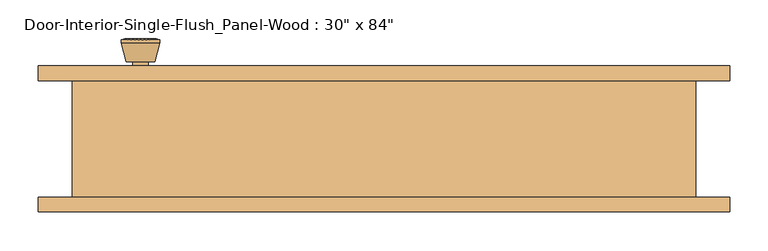
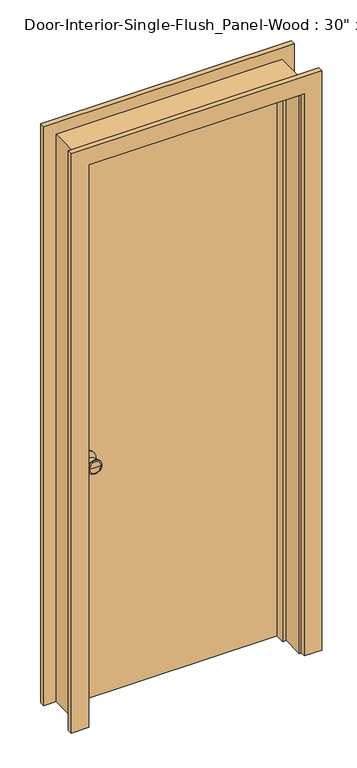
"""IFC4 building model written with IfcOpenShell, lengths in millimetres: door geometry."""

from ifc_helpers import new_model, si_unit, point, frame, frame_2d, origin, origin_with_axes, place, context, project, spatial, polyline, circle_curve, trimmed, segment, composite_curve, outline, extrude, faceted_brep, source, transform, mapped, element, save
from ifc_brep_helpers import plane_surface, cylinder_surface, revolved_surface, advanced_brep


def door_160b0797(model_context):
    return source(origin(), model_context, "Body", "SolidModel", [
        advanced_brep(
        [(-317.5, 32.1, 914.4), (-307.5, 32.1, 914.4), (-327.5, 32.1, 914.4), (-297.0241324, -16.9, 914.4), (-317.5, -16.9, 914.4), (-337.9758676, -16.9, 914.4), (-292.5, -15.0721319, 914.4), (-342.5, -15.0721319, 914.4), (-292.5, -11.6084537, 914.4), (-342.5, -11.6084537, 914.4), (-298.863764, 13.1, 914.4), (-336.136236, 13.1, 914.4), (-307.5, 13.1, 914.4), (-327.5, 13.1, 914.4)],
        [
            (0, 1),
            (1, 2, circle_curve(frame((-317.5, 32.1, 914.4), z_axis=(0.0, 1.0, 0.0), x_axis=(-1.0, 0.0, 0.0)), 10.0)),
            (2, 0),
            (2, 1, circle_curve(frame((-317.5, 32.1, 914.4), z_axis=(0.0, 1.0, 0.0), x_axis=(-1.0, 0.0, 0.0)), 10.0)),
            (3, 4),
            (4, 5),
            (5, 3, circle_curve(frame((-317.5, -16.9, 914.4), z_axis=(0.0, -1.0, 0.0), x_axis=(-1.0, 0.0, 0.0)), 20.4758676)),
            (3, 5, circle_curve(frame((-317.5, -16.9, 914.4), z_axis=(0.0, -1.0, 0.0), x_axis=(-1.0, 0.0, 0.0)), 20.4758676)),
            (6, 3),
            (5, 7),
            (7, 6, circle_curve(frame((-317.5, -15.0721319, 914.4), z_axis=(0.0, -1.0, 0.0), x_axis=(-1.0, 0.0, 0.0)), 25.0)),
            (6, 7, circle_curve(frame((-317.5, -15.0721319, 914.4), z_axis=(0.0, -1.0, 0.0), x_axis=(-1.0, 0.0, 0.0)), 25.0)),
            (8, 6),
            (7, 9),
            (9, 8, circle_curve(frame((-317.5, -11.6084537, 914.4), z_axis=(0.0, -1.0, 0.0), x_axis=(-1.0, 0.0, 0.0)), 25.0)),
            (8, 9, circle_curve(frame((-317.5, -11.6084537, 914.4), z_axis=(0.0, -1.0, 0.0), x_axis=(-1.0, 0.0, 0.0)), 25.0)),
            (10, 8),
            (9, 11),
            (11, 10, circle_curve(frame((-317.5, 13.1, 914.4), z_axis=(0.0, -1.0, 0.0), x_axis=(-1.0, 0.0, 0.0)), 18.636236)),
            (10, 11, circle_curve(frame((-317.5, 13.1, 914.4), z_axis=(0.0, -1.0, 0.0), x_axis=(-1.0, 0.0, 0.0)), 18.636236)),
            (12, 10),
            (11, 13),
            (13, 12, circle_curve(frame((-317.5, 13.1, 914.4), z_axis=(0.0, -1.0, 0.0), x_axis=(-1.0, 0.0, 0.0)), 10.0)),
            (12, 13, circle_curve(frame((-317.5, 13.1, 914.4), z_axis=(0.0, -1.0, 0.0), x_axis=(-1.0, 0.0, 0.0)), 10.0)),
            (1, 12),
            (13, 2),
        ],
        [
            plane_surface(frame((-317.5, 32.1, 914.4), z_axis=(0.0, 1.0, 0.0), x_axis=(-1.0, 0.0, 0.0))),
            plane_surface(frame((-317.5, -16.9, 914.4), z_axis=(0.0, -1.0, 0.0), x_axis=(-1.0, 0.0, 0.0))),
            revolved_surface(polyline([(-337.9758676, -16.9, 914.4), (-342.5, -15.0721319, 914.4)]), (-317.5, 32.1, 914.4), (0.0, 1.0, 0.0)),
            cylinder_surface(frame((-317.5, 32.1, 914.4), z_axis=(0.0, 1.0, 0.0), x_axis=(-1.0, 0.0, 0.0)), 25.0),
            revolved_surface(polyline([(-342.5, -11.6084537, 914.4), (-336.136236, 13.1, 914.4)]), (-317.5, 32.1, 914.4), (0.0, 1.0, 0.0)),
            plane_surface(frame((-317.5, 13.1, 914.4), z_axis=(0.0, 1.0, 0.0), x_axis=(-1.0, 0.0, 0.0))),
            cylinder_surface(frame((-317.5, 32.1, 914.4), z_axis=(0.0, 1.0, 0.0), x_axis=(-1.0, 0.0, 0.0)), 10.0),
        ],
        [
            (0, [[1, 2, 3]]),
            (0, [[-3, 4, -1]]),
            (1, [[5, 6, 7]]),
            (1, [[-6, -5, 8]]),
            (2, [[9, -7, 10, 11]]),
            (2, [[-10, -8, -9, 12]]),
            (3, [[13, -11, 14, 15]]),
            (3, [[-14, -12, -13, 16]]),
            (4, [[17, -15, 18, 19]]),
            (4, [[-18, -16, -17, 20]]),
            (5, [[21, -19, 22, 23]]),
            (5, [[-22, -20, -21, 24]]),
            (6, [[25, -23, 26, -2]]),
            (6, [[-26, -24, -25, -4]]),
        ],
    ),
        extrude(outline(composite_curve([segment(trimmed(circle_curve(frame_2d((914.4, -317.5)), 30.0), [point((914.4, -347.5))], [point((914.4, -287.5))], False, "CARTESIAN"), True, "CONTINUOUS"), segment(trimmed(circle_curve(frame_2d((914.4, -317.5)), 30.0), [point((914.4, -287.5))], [point((914.4, -347.5))], False, "CARTESIAN"), True, "CONTINUOUS")], self_intersect=False)), frame((0.0, 32.1, 0.0), z_axis=(0.0, 1.0, 0.0), x_axis=(0.0, 0.0, 1.0)), (0.0, 0.0, 1.0), 6.0),
        advanced_brep(
        [(-317.5, 79.025, 914.4), (-327.5, 79.025, 914.4), (-307.5, 79.025, 914.4), (-297.0241324, 128.025, 914.4), (-337.9758676, 128.025, 914.4), (-317.5, 128.025, 914.4), (-292.5, 126.1971319, 914.4), (-342.5, 126.1971319, 914.4), (-292.5, 122.7334537, 914.4), (-342.5, 122.7334537, 914.4), (-298.863764, 98.025, 914.4), (-336.136236, 98.025, 914.4), (-307.5, 98.025, 914.4), (-327.5, 98.025, 914.4)],
        [
            (0, 1),
            (1, 2, circle_curve(frame((-317.5, 79.025, 914.4), z_axis=(0.0, -1.0, 0.0), x_axis=(-1.0, 0.0, 0.0)), 10.0)),
            (2, 0),
            (2, 1, circle_curve(frame((-317.5, 79.025, 914.4), z_axis=(0.0, -1.0, 0.0), x_axis=(-1.0, 0.0, 0.0)), 10.0)),
            (3, 4, circle_curve(frame((-317.5, 128.025, 914.4), z_axis=(0.0, 1.0, 0.0), x_axis=(-1.0, 0.0, 0.0)), 20.4758676)),
            (4, 5),
            (5, 3),
            (4, 3, circle_curve(frame((-317.5, 128.025, 914.4), z_axis=(0.0, 1.0, 0.0), x_axis=(-1.0, 0.0, 0.0)), 20.4758676)),
            (6, 7, circle_curve(frame((-317.5, 126.1971319, 914.4), z_axis=(0.0, 1.0, 0.0), x_axis=(-1.0, 0.0, 0.0)), 25.0)),
            (7, 4),
            (3, 6),
            (7, 6, circle_curve(frame((-317.5, 126.1971319, 914.4), z_axis=(0.0, 1.0, 0.0), x_axis=(-1.0, 0.0, 0.0)), 25.0)),
            (8, 9, circle_curve(frame((-317.5, 122.7334537, 914.4), z_axis=(0.0, 1.0, 0.0), x_axis=(-1.0, 0.0, 0.0)), 25.0)),
            (9, 7),
            (6, 8),
            (9, 8, circle_curve(frame((-317.5, 122.7334537, 914.4), z_axis=(0.0, 1.0, 0.0), x_axis=(-1.0, 0.0, 0.0)), 25.0)),
            (10, 11, circle_curve(frame((-317.5, 98.025, 914.4), z_axis=(0.0, 1.0, 0.0), x_axis=(-1.0, 0.0, 0.0)), 18.636236)),
            (11, 9),
            (8, 10),
            (11, 10, circle_curve(frame((-317.5, 98.025, 914.4), z_axis=(0.0, 1.0, 0.0), x_axis=(-1.0, 0.0, 0.0)), 18.636236)),
            (12, 13, circle_curve(frame((-317.5, 98.025, 914.4), z_axis=(0.0, 1.0, 0.0), x_axis=(-1.0, 0.0, 0.0)), 10.0)),
            (13, 11),
            (10, 12),
            (13, 12, circle_curve(frame((-317.5, 98.025, 914.4), z_axis=(0.0, 1.0, 0.0), x_axis=(-1.0, 0.0, 0.0)), 10.0)),
            (1, 13),
            (12, 2),
        ],
        [
            plane_surface(frame((-317.5, 79.025, 914.4), z_axis=(0.0, -1.0, 0.0), x_axis=(-1.0, 0.0, 0.0))),
            plane_surface(frame((-317.5, 128.025, 914.4), z_axis=(0.0, 1.0, 0.0), x_axis=(-1.0, 0.0, 0.0))),
            revolved_surface(polyline([(-337.9758676, 128.025, 914.4), (-342.5, 126.1971319, 914.4)]), (-317.5, 79.025, 914.4), (0.0, -1.0, 0.0)),
            cylinder_surface(frame((-317.5, 79.025, 914.4), z_axis=(0.0, -1.0, 0.0), x_axis=(-1.0, 0.0, 0.0)), 25.0),
            revolved_surface(polyline([(-342.5, 122.7334537, 914.4), (-336.136236, 98.025, 914.4)]), (-317.5, 79.025, 914.4), (0.0, -1.0, 0.0)),
            plane_surface(frame((-317.5, 98.025, 914.4), z_axis=(0.0, -1.0, 0.0), x_axis=(-1.0, 0.0, 0.0))),
            cylinder_surface(frame((-317.5, 79.025, 914.4), z_axis=(0.0, -1.0, 0.0), x_axis=(-1.0, 0.0, 0.0)), 10.0),
        ],
        [
            (0, [[1, 2, 3]]),
            (0, [[-3, 4, -1]]),
            (1, [[5, 6, 7]]),
            (1, [[8, -7, -6]]),
            (2, [[9, 10, -5, 11]]),
            (2, [[12, -11, -8, -10]]),
            (3, [[13, 14, -9, 15]]),
            (3, [[16, -15, -12, -14]]),
            (4, [[17, 18, -13, 19]]),
            (4, [[20, -19, -16, -18]]),
            (5, [[21, 22, -17, 23]]),
            (5, [[24, -23, -20, -22]]),
            (6, [[-2, 25, -21, 26]]),
            (6, [[-4, -26, -24, -25]]),
        ],
    ),
        extrude(outline(composite_curve([segment(trimmed(circle_curve(frame_2d((914.4, -317.5)), 30.0), [point((914.4, -347.5))], [point((914.4, -287.5))], False, "CARTESIAN"), True, "CONTINUOUS"), segment(trimmed(circle_curve(frame_2d((914.4, -317.5)), 30.0), [point((914.4, -287.5))], [point((914.4, -347.5))], False, "CARTESIAN"), True, "CONTINUOUS")], self_intersect=False)), frame((0.0, 73.025, 0.0), z_axis=(0.0, 1.0, 0.0), x_axis=(0.0, 0.0, 1.0)), (0.0, 0.0, 1.0), 6.0),
        extrude(outline(polyline([(381.0, 38.1), (-381.0, 38.1), (-381.0, 73.025), (381.0, 73.025), (381.0, 38.1)])), origin_with_axes(), (0.0, 0.0, 1.0), 2133.6),
        faceted_brep([(406.4, 73.025, 0.0), (406.4, -79.375, 0.0), (381.0, -79.375, 0.0), (381.0, 3.175, 0.0), (368.3, 3.175, 0.0), (368.3, 38.1, 0.0), (381.0, 38.1, 0.0), (381.0, 73.025, 0.0), (406.4, 73.025, 2159.0), (406.4, -79.375, 2159.0), (-406.4, -79.375, 2159.0), (-406.4, -79.375, 0.0), (-381.0, -79.375, 0.0), (-381.0, -79.375, 2133.6), (381.0, -79.375, 2133.6), (381.0, 3.175, 2133.6), (-381.0, 3.175, 2133.6), (-381.0, 3.175, 0.0), (-368.3, 3.175, 0.0), (-368.3, 3.175, 2120.9), (368.3, 3.175, 2120.9), (368.3, 38.1, 2120.9), (-368.3, 38.1, 2120.9), (-368.3, 38.1, 0.0), (-381.0, 38.1, 0.0), (-381.0, 38.1, 2133.6), (381.0, 38.1, 2133.6), (381.0, 73.025, 2133.6), (-381.0, 73.025, 2133.6), (-381.0, 73.025, 0.0), (-406.4, 73.025, 0.0), (-406.4, 73.025, 2159.0)], [[[0, 1, 2, 3, 4, 5, 6, 7]], [[1, 0, 8, 9]], [[2, 1, 9, 10, 11, 12, 13, 14]], [[3, 2, 14, 15]], [[4, 3, 15, 16, 17, 18, 19, 20]], [[5, 4, 20, 21]], [[6, 5, 21, 22, 23, 24, 25, 26]], [[7, 6, 26, 27]], [[0, 7, 27, 28, 29, 30, 31, 8]], [[9, 8, 31, 10]], [[15, 14, 13, 16]], [[21, 20, 19, 22]], [[27, 26, 25, 28]], [[30, 29, 24, 23, 18, 17, 12, 11]], [[10, 31, 30, 11]], [[16, 13, 12, 17]], [[22, 19, 18, 23]], [[28, 25, 24, 29]]]),
        extrude(outline(polyline([(0.0, 387.35), (0.0, 450.85), (2203.45, 450.85), (2203.45, -450.85), (0.0, -450.85), (0.0, -387.35), (2139.95, -387.35), (2139.95, 387.35), (0.0, 387.35)])), frame((0.0, -98.425, 0.0), z_axis=(0.0, 1.0, 0.0), x_axis=(0.0, 0.0, 1.0)), (0.0, 0.0, 1.0), 19.05),
        extrude(outline(polyline([(0.0, 387.35), (0.0, 450.85), (2203.45, 450.85), (2203.45, -450.85), (0.0, -450.85), (0.0, -387.35), (2139.95, -387.35), (2139.95, 387.35), (0.0, 387.35)])), frame((0.0, 73.025, 0.0), z_axis=(0.0, 1.0, 0.0), x_axis=(0.0, 0.0, 1.0)), (0.0, 0.0, 1.0), 19.05),
    ])


if __name__ == "__main__":
    model = new_model("IFC4")
    model_context = context("Model", 3, world=origin())
    ifc_project = project(units=[si_unit("LENGTHUNIT", "METRE", prefix="MILLI")], contexts=[model_context])
    site = spatial("IfcSite", under=ifc_project)
    building = spatial("IfcBuilding", under=site)
    placement = place(None, origin())
    door_shape = door_160b0797(model_context)
    element("IfcDoor", 1, ObjectType="Door-Interior-Single-Flush_Panel-Wood : 30\" x 84\"", at=placement, inside=building, context=model_context, shape_type="MappedRepresentation", body=[
        mapped(door_shape, transform((0.0, 0.0, 0.0), x_axis=(1.0, 0.0, 0.0), y_axis=(0.0, 1.0, 0.0), z_axis=(0.0, 0.0, 1.0))),
    ])
    save(model, "model.ifc")

# Revit data of these elements
# Type "Door-Interior-Single-Flush_Panel-Wood : 30\" x 84\""
#   Type Mark = "12"
#   Assembly Code = "C1020300"
#   Analytic Construction = "Wooden"
#   Thickness = 0' - 1 3/8"
#   Thermal Resistance (R) = 2.5876 (h·ft²·°F)/BTU
#   Swing Angle [instance default] = 90.00°
#   Rough Width = 2' - 8"
#   Rough Height = 7' - 1"
#   Height = 7' - 0"
#   Width = 2' - 6"
#   Heat Transfer Coefficient (U) = 0.3865 BTU/(h·ft²·°F)
#   Trim Material = Cherry
#   Panel Material = Cherry
#   Frame Material = Cherry
#   Door Handle Material = Aluminum
#   Visual Light Transmittance = 0
#   Solar Heat Gain Coefficient = 0
#   Wall Closure = (empty or 0)
#   Function = (empty or 0)
# Element 1 (IfcDoor, "Door-Interior-Single-Flush_Panel-Wood : 30\" x 84\"")
#   Materials on its faces: "Cherry", "Aluminum"
# Materials
#   "Cherry": class "Wood", colour RGB 226 177 128, transparency 0, Description = "Prunus Serotina", Cost = 0
#   "Aluminum": class "Metal", colour RGB 247 247 247, transparency 0, Description = "Aluminum 6061", Cost = 0
